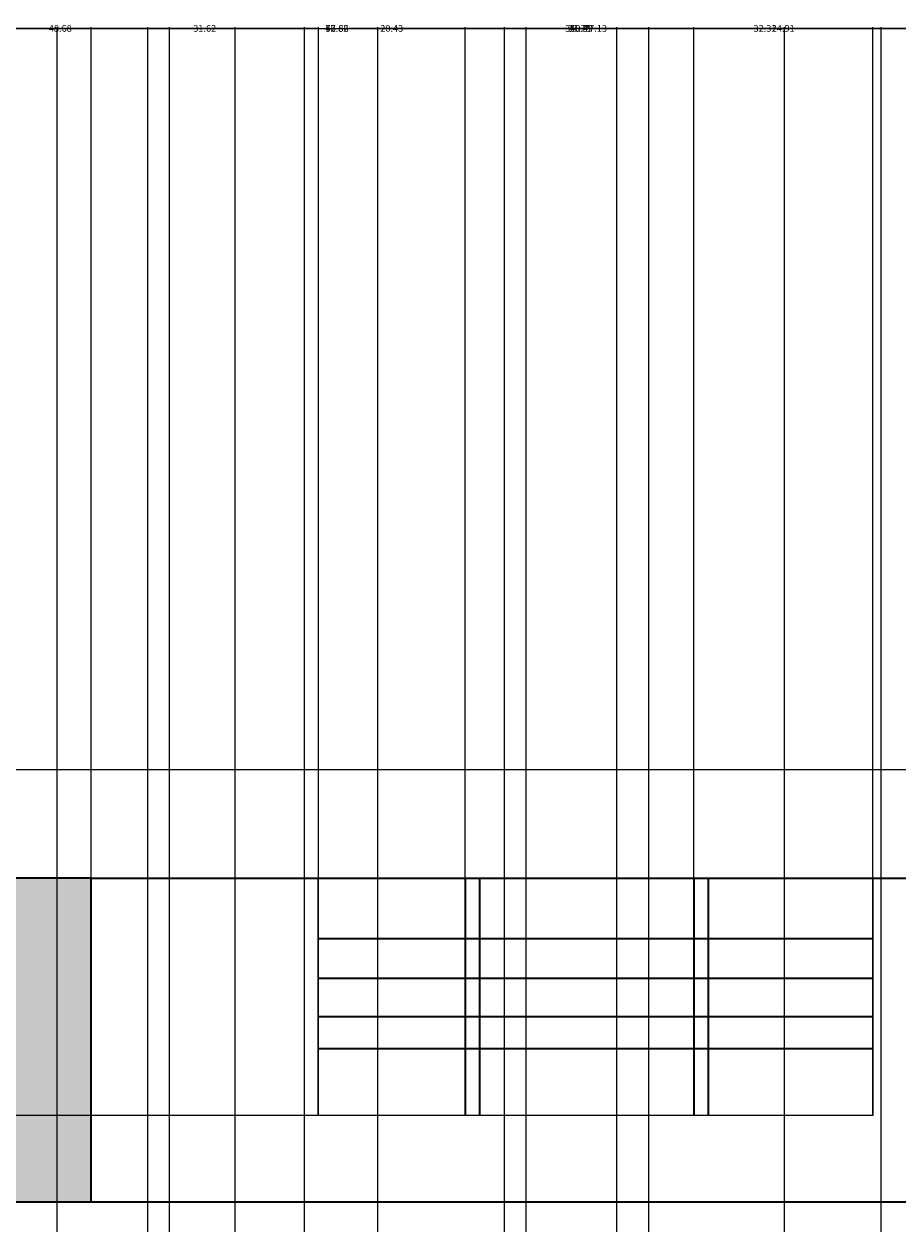
# Model space of a CAD drawing. Units: inches. Extents: x -5 to 714, y 84 to 644.
# Tile 13 of 20: x 220 to 342, y 477 to 644. Entities that reach past the tile are written whole.
import ezdxf

# ---------------------------------------------------------------- set-up
doc = ezdxf.new("R2010")
doc.units = ezdxf.units.IN
doc.header["$MEASUREMENT"] = 0
for name, color, linetype, lineweight in [('A-ANNO-DIMS', 2, 'Continuous', 18), ('A-ELEV', 7, 'Continuous', 35), ('A-ELEV-PATT', 8, 'Continuous', 13), ('A-GLAZ', 3, 'Continuous', 25)]:
    doc.layers.add(name, color=color, linetype=linetype, lineweight=lineweight)
doc.styles.get("Standard").update_dxf_attribs({"font": 'arial.ttf'})
doc.dimstyles.get("Standard").update_dxf_attribs({"dimtxt": 0.9375, "dimasz": 0.18, "dimexe": 0.18, "dimexo": 0.0625, "dimgap": 0.09, "dimtad": 0, "dimtih": 1, "dimtoh": 1, "dimdec": 4, "dimzin": 0, "dimdsep": 46, "dimlunit": 4, "dimtxsty": 'Standard', "dimcen": 0.09, "dimadec": 0, "dimazin": 0, "dimtfac": 1, "dimtdec": 4, "dimtofl": 0, "dimtmove": 0, "dimatfit": 3, "dimfxl": 1, "dimtolj": 1, "dimtzin": 0, "dimarcsym": 0})

# ---------------------------------------------------------------- blocks, each defined once
blk = doc.blocks.new('*D11')
at = {"layer": 'A-ANNO-DIMS', "color": 0, "lineweight": -2, "transparency": 16777216}
for p, q in [((198.38, 525.26), (198.38, 643.61)), ((198.56, 643.43), (211.83, 643.43)), ((229.18, 643.43), (215.91, 643.43)), ((229.36, 525.26), (229.36, 643.61))]:
    blk.add_line(p, q, dxfattribs=at)
at = {"layer": 'A-ANNO-DIMS', "color": 0, "transparency": 16777216}
for points in [[(198.56, 643.46), (198.56, 643.4), (198.38, 643.43)], [(229.18, 643.46), (229.18, 643.4), (229.36, 643.43)]]:
    blk.add_solid(points, dxfattribs=at)
at = {"layer": 'Defpoints', "color": 0, "transparency": 16777216}
for p in [(229.36, 643.43), (198.38, 525.19), (229.36, 525.19)]:
    blk.add_point(p, dxfattribs=at)
at = {"layer": 'A-ANNO-DIMS', "color": 0, "transparency": 16777216, "insert": (213.87, 643.43), "char_height": 0.938, "attachment_point": 5}
blk.add_mtext('\\A1;30.975', dxfattribs=at)
blk = doc.blocks.new('*D12')
at = {"layer": 'A-ANNO-DIMS', "color": 0, "lineweight": -2, "transparency": 16777216}
for p, q in [((229.36, 525.26), (229.36, 643.61)), ((229.54, 643.43), (243.5, 643.43)), ((260.8, 643.43), (246.83, 643.43)), ((260.98, 525.26), (260.98, 643.61))]:
    blk.add_line(p, q, dxfattribs=at)
at = {"layer": 'A-ANNO-DIMS', "color": 0, "transparency": 16777216}
for points in [[(229.54, 643.46), (229.54, 643.4), (229.36, 643.43)], [(260.8, 643.46), (260.8, 643.4), (260.98, 643.43)]]:
    blk.add_solid(points, dxfattribs=at)
at = {"layer": 'Defpoints', "color": 0, "transparency": 16777216}
for p in [(260.98, 643.43), (229.36, 525.19), (260.98, 525.19)]:
    blk.add_point(p, dxfattribs=at)
at = {"layer": 'A-ANNO-DIMS', "color": 0, "transparency": 16777216, "insert": (245.17, 643.43), "char_height": 0.938, "attachment_point": 5}
blk.add_mtext('\\A1;31.62', dxfattribs=at)
blk = doc.blocks.new('*D13')
at = {"layer": 'A-ANNO-DIMS', "color": 0, "lineweight": -2, "transparency": 16777216}
for p, q in [((260.98, 525.26), (260.98, 643.61)), ((261.16, 643.43), (297.87, 643.43)), ((337.93, 643.43), (301.21, 643.43)), ((338.11, 525.26), (338.11, 643.61))]:
    blk.add_line(p, q, dxfattribs=at)
at = {"layer": 'A-ANNO-DIMS', "color": 0, "transparency": 16777216}
for points in [[(261.16, 643.46), (261.16, 643.4), (260.98, 643.43)], [(337.93, 643.46), (337.93, 643.4), (338.11, 643.43)]]:
    blk.add_solid(points, dxfattribs=at)
at = {"layer": 'Defpoints', "color": 0, "transparency": 16777216}
for p in [(338.11, 643.43), (260.98, 525.19), (338.11, 525.19)]:
    blk.add_point(p, dxfattribs=at)
at = {"layer": 'A-ANNO-DIMS', "color": 0, "transparency": 16777216, "insert": (299.54, 643.43), "char_height": 0.938, "attachment_point": 5}
blk.add_mtext('\\A1;77.13', dxfattribs=at)
blk = doc.blocks.new('*D14')
at = {"layer": 'A-ANNO-DIMS', "color": 0, "lineweight": -2, "transparency": 16777216}
for p, q in [((338.11, 525.26), (338.11, 643.61)), ((338.29, 643.43), (349.15, 643.43)), ((364.1, 643.43), (353.24, 643.43)), ((364.28, 525.26), (364.28, 643.61))]:
    blk.add_line(p, q, dxfattribs=at)
at = {"layer": 'A-ANNO-DIMS', "color": 0, "transparency": 16777216}
for points in [[(338.29, 643.46), (338.29, 643.4), (338.11, 643.43)], [(364.1, 643.46), (364.1, 643.4), (364.28, 643.43)]]:
    blk.add_solid(points, dxfattribs=at)
at = {"layer": 'Defpoints', "color": 0, "transparency": 16777216}
for p in [(364.28, 643.43), (338.11, 525.19), (364.28, 525.19)]:
    blk.add_point(p, dxfattribs=at)
at = {"layer": 'A-ANNO-DIMS', "color": 0, "transparency": 16777216, "insert": (351.19, 643.43), "char_height": 0.938, "attachment_point": 5}
blk.add_mtext('\\A1;26.175', dxfattribs=at)
blk = doc.blocks.new('*D16')
at = {"layer": 'A-ANNO-DIMS', "color": 0, "lineweight": -2, "transparency": 16777216}
for p, q in [((364.22, 540.29), (-2.74, 540.29)), ((-2.56, 540.11), (-2.56, 510.8)), ((-2.56, 480.35), (-2.56, 509.66)), ((364.22, 480.17), (-2.74, 480.17))]:
    blk.add_line(p, q, dxfattribs=at)
at = {"layer": 'A-ANNO-DIMS', "color": 0, "transparency": 16777216}
for points in [[(-2.59, 540.11), (-2.53, 540.11), (-2.56, 540.29)], [(-2.59, 480.35), (-2.53, 480.35), (-2.56, 480.17)]]:
    blk.add_solid(points, dxfattribs=at)
at = {"layer": 'Defpoints', "color": 0, "transparency": 16777216}
for p in [(-2.56, 540.29), (364.28, 540.29), (364.28, 480.17)]:
    blk.add_point(p, dxfattribs=at)
at = {"layer": 'A-ANNO-DIMS', "color": 0, "transparency": 16777216, "insert": (-2.56, 510.23), "char_height": 0.938, "attachment_point": 5}
blk.add_mtext('\\A1;60.11', dxfattribs=at)
blk = doc.blocks.new('*D17')
at = {"layer": 'A-ANNO-DIMS', "color": 0, "lineweight": -2, "transparency": 16777216}
for p, q in [((338.04, 525.19), (-2.74, 525.19)), ((-2.56, 525.01), (-2.56, 509.25)), ((-2.56, 492.35), (-2.56, 508.11)), ((338.04, 492.17), (-2.74, 492.17))]:
    blk.add_line(p, q, dxfattribs=at)
at = {"layer": 'A-ANNO-DIMS', "color": 0, "transparency": 16777216}
for points in [[(-2.59, 525.01), (-2.53, 525.01), (-2.56, 525.19)], [(-2.59, 492.35), (-2.53, 492.35), (-2.56, 492.17)]]:
    blk.add_solid(points, dxfattribs=at)
at = {"layer": 'Defpoints', "color": 0, "transparency": 16777216}
for p in [(-2.56, 525.19), (338.11, 525.19), (338.11, 492.17)]:
    blk.add_point(p, dxfattribs=at)
at = {"layer": 'A-ANNO-DIMS', "color": 0, "transparency": 16777216, "insert": (-2.56, 508.68), "char_height": 0.938, "attachment_point": 5}
blk.add_mtext('\\A1;33.03', dxfattribs=at)
blk = doc.blocks.new('*D18')
at = {"layer": 'A-ANNO-DIMS', "color": 0, "lineweight": -2, "transparency": 16777216}
for p, q in [((260.98, 492.23), (260.98, 643.61)), ((261.16, 643.43), (269.51, 643.43)), ((281.23, 643.43), (272.87, 643.43)), ((281.41, 492.23), (281.41, 643.61))]:
    blk.add_line(p, q, dxfattribs=at)
at = {"layer": 'A-ANNO-DIMS', "color": 0, "transparency": 16777216}
for points in [[(261.16, 643.46), (261.16, 643.4), (260.98, 643.43)], [(281.23, 643.46), (281.23, 643.4), (281.41, 643.43)]]:
    blk.add_solid(points, dxfattribs=at)
at = {"layer": 'Defpoints', "color": 0, "transparency": 16777216}
for p in [(281.41, 643.43), (260.98, 492.17), (281.41, 492.17)]:
    blk.add_point(p, dxfattribs=at)
at = {"layer": 'A-ANNO-DIMS', "color": 0, "transparency": 16777216, "insert": (271.19, 643.43), "char_height": 0.938, "attachment_point": 5}
blk.add_mtext('\\A1;20.43', dxfattribs=at)
blk = doc.blocks.new('*D19')
at = {"layer": 'A-ANNO-DIMS', "color": 0, "lineweight": -2, "transparency": 16777216}
for p, q in [((281.41, 492.23), (281.41, 643.61)), ((281.59, 643.43), (295.63, 643.43)), ((313.02, 643.43), (298.98, 643.43)), ((313.2, 492.23), (313.2, 643.61))]:
    blk.add_line(p, q, dxfattribs=at)
at = {"layer": 'A-ANNO-DIMS', "color": 0, "transparency": 16777216}
for points in [[(281.59, 643.46), (281.59, 643.4), (281.41, 643.43)], [(313.02, 643.46), (313.02, 643.4), (313.2, 643.43)]]:
    blk.add_solid(points, dxfattribs=at)
at = {"layer": 'Defpoints', "color": 0, "transparency": 16777216}
for p in [(313.2, 643.43), (281.41, 492.17), (313.2, 492.17)]:
    blk.add_point(p, dxfattribs=at)
at = {"layer": 'A-ANNO-DIMS', "color": 0, "transparency": 16777216, "insert": (297.3, 643.43), "char_height": 0.938, "attachment_point": 5}
blk.add_mtext('\\A1;31.79', dxfattribs=at)
blk = doc.blocks.new('*D20')
at = {"layer": 'A-ANNO-DIMS', "color": 0, "lineweight": -2, "transparency": 16777216}
for p, q in [((313.2, 492.23), (313.2, 643.61)), ((313.38, 643.43), (324.06, 643.43)), ((337.93, 643.43), (327.24, 643.43)), ((338.11, 492.23), (338.11, 643.61))]:
    blk.add_line(p, q, dxfattribs=at)
at = {"layer": 'A-ANNO-DIMS', "color": 0, "transparency": 16777216}
for points in [[(313.38, 643.46), (313.38, 643.4), (313.2, 643.43)], [(337.93, 643.46), (337.93, 643.4), (338.11, 643.43)]]:
    blk.add_solid(points, dxfattribs=at)
at = {"layer": 'Defpoints', "color": 0, "transparency": 16777216}
for p in [(338.11, 643.43), (313.2, 492.17), (338.11, 492.17)]:
    blk.add_point(p, dxfattribs=at)
at = {"layer": 'A-ANNO-DIMS', "color": 0, "transparency": 16777216, "insert": (325.65, 643.43), "char_height": 0.938, "attachment_point": 5}
blk.add_mtext('\\A1;24.91', dxfattribs=at)
blk = doc.blocks.new('*D23')
at = {"layer": 'A-ANNO-DIMS', "color": 0, "lineweight": -2, "transparency": 16777216}
for p, q in [((229.3, 525.19), (-2.74, 525.19)), ((-2.56, 525.01), (-2.56, 503.25)), ((-2.56, 480.35), (-2.56, 502.11)), ((229.3, 480.17), (-2.74, 480.17))]:
    blk.add_line(p, q, dxfattribs=at)
at = {"layer": 'A-ANNO-DIMS', "color": 0, "transparency": 16777216}
for points in [[(-2.59, 525.01), (-2.53, 525.01), (-2.56, 525.19)], [(-2.59, 480.35), (-2.53, 480.35), (-2.56, 480.17)]]:
    blk.add_solid(points, dxfattribs=at)
at = {"layer": 'Defpoints', "color": 0, "transparency": 16777216}
for p in [(-2.56, 525.19), (229.36, 525.19), (229.36, 480.17)]:
    blk.add_point(p, dxfattribs=at)
at = {"layer": 'A-ANNO-DIMS', "color": 0, "transparency": 16777216, "insert": (-2.56, 502.68), "char_height": 0.938, "attachment_point": 5}
blk.add_mtext('\\A1;45.02', dxfattribs=at)
blk = doc.blocks.new('*D24')
at = {"layer": 'A-ANNO-DIMS', "color": 0, "lineweight": -2, "transparency": 16777216}
for p, q in [((126.73, 480.23), (126.73, 643.61)), ((126.91, 643.43), (295.25, 643.43)), ((466.92, 643.43), (298.58, 643.43)), ((467.1, 480.23), (467.1, 643.61))]:
    blk.add_line(p, q, dxfattribs=at)
at = {"layer": 'A-ANNO-DIMS', "color": 0, "transparency": 16777216}
for points in [[(126.91, 643.46), (126.91, 643.4), (126.73, 643.43)], [(466.92, 643.46), (466.92, 643.4), (467.1, 643.43)]]:
    blk.add_solid(points, dxfattribs=at)
at = {"layer": 'Defpoints', "color": 0, "transparency": 16777216}
for p in [(467.1, 643.43), (126.73, 480.17), (467.1, 480.17)]:
    blk.add_point(p, dxfattribs=at)
at = {"layer": 'A-ANNO-DIMS', "color": 0, "transparency": 16777216, "insert": (296.91, 643.43), "char_height": 0.938, "attachment_point": 5}
blk.add_mtext('\\A1;340.4', dxfattribs=at)
blk = doc.blocks.new('*D31')
at = {"layer": 'A-ANNO-DIMS', "color": 0, "lineweight": -2, "transparency": 16777216}
for p, q in [((135.73, 345.26), (135.73, 643.61)), ((135.91, 643.43), (184.51, 643.43)), ((237.09, 643.43), (188.49, 643.43)), ((237.27, 345.26), (237.27, 643.61))]:
    blk.add_line(p, q, dxfattribs=at)
at = {"layer": 'A-ANNO-DIMS', "color": 0, "transparency": 16777216}
for points in [[(135.91, 643.46), (135.91, 643.4), (135.73, 643.43)], [(237.09, 643.46), (237.09, 643.4), (237.27, 643.43)]]:
    blk.add_solid(points, dxfattribs=at)
at = {"layer": 'Defpoints', "color": 0, "transparency": 16777216}
for p in [(237.27, 643.43), (135.73, 345.19), (237.27, 345.19)]:
    blk.add_point(p, dxfattribs=at)
at = {"layer": 'A-ANNO-DIMS', "color": 0, "transparency": 16777216, "insert": (186.5, 643.43), "char_height": 0.938, "attachment_point": 5}
blk.add_mtext('\\A1;101.54', dxfattribs=at)
blk = doc.blocks.new('*D32')
at = {"layer": 'A-ANNO-DIMS', "color": 0, "lineweight": -2, "transparency": 16777216}
for p, q in [((237.27, 417.15), (237.27, 643.61)), ((237.45, 643.43), (261.91, 643.43)), ((289.7, 643.43), (265.24, 643.43)), ((289.88, 417.15), (289.88, 643.61))]:
    blk.add_line(p, q, dxfattribs=at)
at = {"layer": 'A-ANNO-DIMS', "color": 0, "transparency": 16777216}
for points in [[(237.45, 643.46), (237.45, 643.4), (237.27, 643.43)], [(289.7, 643.46), (289.7, 643.4), (289.88, 643.43)]]:
    blk.add_solid(points, dxfattribs=at)
at = {"layer": 'Defpoints', "color": 0, "transparency": 16777216}
for p in [(289.88, 643.43), (237.27, 417.09), (289.88, 417.09)]:
    blk.add_point(p, dxfattribs=at)
at = {"layer": 'A-ANNO-DIMS', "color": 0, "transparency": 16777216, "insert": (263.57, 643.43), "char_height": 0.938, "attachment_point": 5}
blk.add_mtext('\\A1;52.62', dxfattribs=at)
blk = doc.blocks.new('*D33')
at = {"layer": 'A-ANNO-DIMS', "color": 0, "lineweight": -2, "transparency": 16777216}
for p, q in [((240.27, 348.26), (240.27, 643.61)), ((240.45, 643.43), (261.89, 643.43)), ((286.7, 643.43), (265.26, 643.43)), ((286.88, 348.26), (286.88, 643.61))]:
    blk.add_line(p, q, dxfattribs=at)
at = {"layer": 'A-ANNO-DIMS', "color": 0, "transparency": 16777216}
for points in [[(240.45, 643.46), (240.45, 643.4), (240.27, 643.43)], [(286.7, 643.46), (286.7, 643.4), (286.88, 643.43)]]:
    blk.add_solid(points, dxfattribs=at)
at = {"layer": 'Defpoints', "color": 0, "transparency": 16777216}
for p in [(286.88, 643.43), (240.27, 348.19), (286.88, 348.19)]:
    blk.add_point(p, dxfattribs=at)
at = {"layer": 'A-ANNO-DIMS', "color": 0, "transparency": 16777216, "insert": (263.57, 643.43), "char_height": 0.938, "attachment_point": 5}
blk.add_mtext('\\A1;46.62', dxfattribs=at)
blk = doc.blocks.new('*D36')
at = {"layer": 'A-ANNO-DIMS', "color": 0, "lineweight": -2, "transparency": 16777216}
for p, q in [((224.64, 426.51), (224.64, 643.61)), ((224.82, 643.43), (261.91, 643.43)), ((302.32, 643.43), (265.24, 643.43)), ((302.5, 426.51), (302.5, 643.61))]:
    blk.add_line(p, q, dxfattribs=at)
at = {"layer": 'A-ANNO-DIMS', "color": 0, "transparency": 16777216}
for points in [[(224.82, 643.46), (224.82, 643.4), (224.64, 643.43)], [(302.32, 643.46), (302.32, 643.4), (302.5, 643.43)]]:
    blk.add_solid(points, dxfattribs=at)
at = {"layer": 'Defpoints', "color": 0, "transparency": 16777216}
for p in [(302.5, 643.43), (224.64, 426.45), (302.5, 426.45)]:
    blk.add_point(p, dxfattribs=at)
at = {"layer": 'A-ANNO-DIMS', "color": 0, "transparency": 16777216, "insert": (263.57, 643.43), "char_height": 0.938, "attachment_point": 5}
blk.add_mtext('\\A1;77.86', dxfattribs=at)
blk = doc.blocks.new('*D51')
at = {"layer": 'A-ANNO-DIMS', "color": 0, "lineweight": -2, "transparency": 16777216}
for p, q in [((200.74, 201.26), (200.74, 643.61)), ((200.92, 643.43), (223.39, 643.43)), ((249.24, 643.43), (226.77, 643.43)), ((249.42, 201.26), (249.42, 643.61))]:
    blk.add_line(p, q, dxfattribs=at)
at = {"layer": 'A-ANNO-DIMS', "color": 0, "transparency": 16777216}
for points in [[(200.92, 643.46), (200.92, 643.4), (200.74, 643.43)], [(249.24, 643.46), (249.24, 643.4), (249.42, 643.43)]]:
    blk.add_solid(points, dxfattribs=at)
at = {"layer": 'Defpoints', "color": 0, "transparency": 16777216}
for p in [(249.42, 643.43), (200.74, 201.19), (249.42, 201.19)]:
    blk.add_point(p, dxfattribs=at)
at = {"layer": 'A-ANNO-DIMS', "color": 0, "transparency": 16777216, "insert": (225.08, 643.43), "char_height": 0.938, "attachment_point": 5}
blk.add_mtext('\\A1;48.68', dxfattribs=at)
blk = doc.blocks.new('*D54')
at = {"layer": 'A-ANNO-DIMS', "color": 0, "lineweight": -2, "transparency": 16777216}
for p, q in [((259.07, 315.16), (259.07, 643.61)), ((259.25, 643.43), (424.21, 643.43)), ((593.25, 643.43), (428.28, 643.43)), ((593.43, 315.16), (593.43, 643.61))]:
    blk.add_line(p, q, dxfattribs=at)
at = {"layer": 'A-ANNO-DIMS', "color": 0, "transparency": 16777216}
for points in [[(259.25, 643.46), (259.25, 643.4), (259.07, 643.43)], [(593.25, 643.46), (593.25, 643.4), (593.43, 643.43)]]:
    blk.add_solid(points, dxfattribs=at)
at = {"layer": 'Defpoints', "color": 0, "transparency": 16777216}
for p in [(593.43, 643.43), (259.07, 315.1), (593.43, 315.1)]:
    blk.add_point(p, dxfattribs=at)
at = {"layer": 'A-ANNO-DIMS', "color": 0, "transparency": 16777216, "insert": (426.25, 643.43), "char_height": 0.938, "attachment_point": 5}
blk.add_mtext('\\A1;334.36', dxfattribs=at)
blk = doc.blocks.new('*D60')
at = {"layer": 'A-ANNO-DIMS', "color": 0, "lineweight": -2, "transparency": 16777216}
for p, q in [((269.24, 277.11), (269.24, 643.61)), ((269.42, 643.43), (295.86, 643.43)), ((325.65, 643.43), (299.21, 643.43)), ((325.83, 266.06), (325.83, 643.61))]:
    blk.add_line(p, q, dxfattribs=at)
at = {"layer": 'A-ANNO-DIMS', "color": 0, "transparency": 16777216}
for points in [[(269.42, 643.46), (269.42, 643.4), (269.24, 643.43)], [(325.65, 643.46), (325.65, 643.4), (325.83, 643.43)]]:
    blk.add_solid(points, dxfattribs=at)
at = {"layer": 'Defpoints', "color": 0, "transparency": 16777216}
for p in [(325.83, 643.43), (269.24, 277.05), (325.83, 266)]:
    blk.add_point(p, dxfattribs=at)
at = {"layer": 'A-ANNO-DIMS', "color": 0, "transparency": 16777216, "insert": (297.54, 643.43), "char_height": 0.938, "attachment_point": 5}
blk.add_mtext('\\A1;56.59', dxfattribs=at)
blk = doc.blocks.new('*D61')
at = {"layer": 'A-ANNO-DIMS', "color": 0, "lineweight": -2, "transparency": 16777216}
for p, q in [((325.83, 266.06), (325.83, 643.61)), ((326.01, 643.43), (364.93, 643.43)), ((407.2, 643.43), (368.28, 643.43)), ((407.38, 266.06), (407.38, 643.61))]:
    blk.add_line(p, q, dxfattribs=at)
at = {"layer": 'A-ANNO-DIMS', "color": 0, "transparency": 16777216}
for points in [[(326.01, 643.46), (326.01, 643.4), (325.83, 643.43)], [(407.2, 643.46), (407.2, 643.4), (407.38, 643.43)]]:
    blk.add_solid(points, dxfattribs=at)
at = {"layer": 'Defpoints', "color": 0, "transparency": 16777216}
for p in [(407.38, 643.43), (325.83, 266), (407.38, 266)]:
    blk.add_point(p, dxfattribs=at)
at = {"layer": 'A-ANNO-DIMS', "color": 0, "transparency": 16777216, "insert": (366.61, 643.43), "char_height": 0.938, "attachment_point": 5}
blk.add_mtext('\\A1;81.55', dxfattribs=at)
blk = doc.blocks.new('*D83')
at = {"layer": 'A-ANNO-DIMS', "color": 0, "lineweight": -2, "transparency": 16777216}
for p, q in [((306.96, 144.93), (306.96, 643.61)), ((307.14, 643.43), (321.53, 643.43)), ((339.09, 643.43), (324.69, 643.43)), ((339.27, 144.93), (339.27, 643.61))]:
    blk.add_line(p, q, dxfattribs=at)
at = {"layer": 'A-ANNO-DIMS', "color": 0, "transparency": 16777216}
for points in [[(307.14, 643.46), (307.14, 643.4), (306.96, 643.43)], [(339.09, 643.46), (339.09, 643.4), (339.27, 643.43)]]:
    blk.add_solid(points, dxfattribs=at)
at = {"layer": 'Defpoints', "color": 0, "transparency": 16777216}
for p in [(339.27, 643.43), (306.96, 144.86), (339.27, 144.86)]:
    blk.add_point(p, dxfattribs=at)
at = {"layer": 'A-ANNO-DIMS', "color": 0, "transparency": 16777216, "insert": (323.11, 643.43), "char_height": 0.938, "attachment_point": 5}
blk.add_mtext('\\A1;32.31', dxfattribs=at)

msp = doc.modelspace()

# ---------------------------------------------------------------- hatches: boundary and pattern name
at = {"layer": 'A-ELEV-PATT', "transparency": 33554687}
h = msp.add_hatch(color=256, dxfattribs=at)
h.dxf.hatch_style = 1
h.paths.add_polyline_path([(188.3677, 525.1928), (67.9893, 525.1928), (67.9893, 489.1928), (67.9893, 345.1928), (126.7303, 345.1928), (126.7303, 480.1709), (229.3575, 480.1709), (229.3575, 525.1928), (212.6043, 525.1928), (212.6043, 482.7164), (211.0019, 482.7164), (211.0019, 525.1928), (207.6919, 525.1928), (199.9852, 525.1928), (199.9852, 482.7164), (198.3828, 482.7164), (198.3828, 525.1928), (189.9701, 525.1928), (189.9701, 482.7164), (188.3677, 482.7164)])
h.paths.add_polyline_path([(121.3589, 336.2066), (75.5048, 336.2066), (75.5048, 319.345), (121.3589, 319.345)])
h.paths.add_polyline_path([(121.3589, 319.345), (75.5048, 319.345), (75.5048, 302.3045), (121.3589, 302.3045)])
h.paths.add_polyline_path([(121.3589, 302.3045), (75.5048, 302.3045), (75.5048, 282.8561), (121.3589, 282.8561)])
h.paths.add_polyline_path([(121.3589, 282.8561), (75.5048, 282.8561), (75.5048, 261.5556), (121.3589, 261.5556)])
h.paths.add_polyline_path([(121.3589, 261.5556), (75.5048, 261.5556), (75.5048, 243.7009), (121.3589, 243.7009)])
h.paths.add_polyline_path([(121.3589, 243.7009), (75.5048, 243.7009), (75.5048, 223.5117), (121.3589, 223.5117)])
h.paths.add_polyline_path([(121.3589, 223.5117), (75.5048, 223.5117), (75.5048, 212.5836), (121.3589, 212.5836)])
h.paths.add_polyline_path([(121.3589, 212.5836), (75.5048, 212.5836), (75.5048, 201.1928), (121.3589, 201.1928)])
h.paths.add_polyline_path([(179.9335, 201.1928), (30.1395, 201.1928), (30.1395, 198.7054), (179.9335, 198.7054)])
h.paths.add_polyline_path([(187.6349, 201.1928), (179.9335, 201.1928), (179.9335, 198.7054), (179.9335, 141.1928), (269.2446, 141.1928), (269.2446, 201.1928), (263.4349, 201.1928), (263.4349, 152.1176), (187.6349, 152.1176)])
h.paths.add_polyline_path([(269.2446, 277.0513), (269.2446, 287.501), (269.2446, 306.6286), (578.0915, 306.6286), (578.0915, 201.1928), (593.428, 201.1928), (593.428, 315.0968), (584.4202, 315.0968), (259.0665, 315.0968), (259.0665, 201.1928), (263.4349, 201.1928), (269.2446, 201.1928)])

# ---------------------------------------------------------------- linework, layer by layer
at = {"layer": 'A-ELEV'}
for p, q in [((229.3575, 525.1928), (207.6919, 525.1928)), ((229.3575, 480.1709), (229.3575, 525.1928)), ((229.3575, 525.1928), (364.2809, 525.1928)), ((281.4098, 525.1928), (281.4098, 492.1651)), ((283.4098, 525.1928), (283.4098, 492.1651)), ((313.1984, 525.1928), (313.1984, 492.1651)), ((315.1984, 525.1928), (315.1984, 492.1651)), ((260.9786, 516.8026), (338.106, 516.8026)), ((260.9786, 511.2941), (338.106, 511.2941)), ((260.9786, 505.9633), (338.106, 505.9633)), ((260.9786, 501.521), (338.106, 501.521)), ((126.7303, 480.1709), (229.3575, 480.1709)), ((229.3575, 480.1709), (467.0994, 480.1709))]:
    msp.add_line(p, q, dxfattribs=at)
at = {"layer": 'A-GLAZ'}
msp.add_lwpolyline([(260.9786, 525.1928), (338.106, 525.1928), (338.106, 492.1651), (260.9786, 492.1651)], close=True, dxfattribs=at)

# ---------------------------------------------------------------- dimensions: what is measured, and where the dimension line sits
at = {"layer": 'A-ANNO-DIMS'}
for base, p1, p2, override, picture, middle in [((467.0994, 643.4276), (126.7303, 480.1709), (467.0994, 480.1709), {"dimdec": 1, "dimlfac": 1, "dimrnd": 0, "dimzin": 0, "dimdsep": 46, "dimlunit": 2}, '*D24', (296.9148, 643.4276)), ((237.2654, 643.4276), (135.7303, 345.1928), (237.2654, 345.1928), {"dimdec": 2, "dimlfac": 1, "dimrnd": 0, "dimzin": 0, "dimdsep": 46, "dimlunit": 2}, '*D31', (186.4978, 643.4276)), ((229.3575, 643.4276), (198.3828, 525.1928), (229.3575, 525.1928), {"dimdec": 3, "dimlfac": 1, "dimrnd": 0, "dimzin": 0, "dimdsep": 46, "dimlunit": 2}, '*D11', (213.8702, 643.4276)), ((249.4181, 643.4276), (200.7361, 201.1928), (249.4181, 201.1928), {"dimdec": 2, "dimlfac": 1, "dimrnd": 0, "dimzin": 0, "dimdsep": 46, "dimlunit": 2}, '*D51', (225.0771, 643.4276)), ((302.5023, 643.4276), (224.6446, 426.4485), (302.5023, 426.4485), {"dimdec": 2, "dimlfac": 1, "dimrnd": 0, "dimzin": 0, "dimdsep": 46, "dimlunit": 2}, '*D36', (263.5734, 643.4276)), ((260.9786, 643.4276), (229.3575, 525.1928), (260.9786, 525.1928), {"dimdec": 2, "dimlfac": 1, "dimrnd": 0, "dimzin": 0, "dimdsep": 46, "dimlunit": 2}, '*D12', (245.1681, 643.4276)), ((289.8815, 643.4276), (237.2654, 417.0908), (289.8815, 417.0908), {"dimdec": 2, "dimlfac": 1, "dimrnd": 0, "dimzin": 0, "dimdsep": 46, "dimlunit": 2}, '*D32', (263.5734, 643.4276)), ((286.8815, 643.4276), (240.2654, 348.1928), (286.8815, 348.1928), {"dimdec": 2, "dimlfac": 1, "dimrnd": 0, "dimzin": 0, "dimdsep": 46, "dimlunit": 2}, '*D33', (263.5734, 643.4276)), ((593.428, 643.4276), (259.0665, 315.0968), (593.428, 315.0968), {"dimdec": 2, "dimlfac": 1, "dimrnd": 0, "dimzin": 0, "dimdsep": 46, "dimlunit": 2}, '*D54', (426.2472, 643.4276)), ((338.106, 643.4276), (260.9786, 525.1928), (338.106, 525.1928), {"dimdec": 2, "dimlfac": 1, "dimrnd": 0, "dimzin": 0, "dimdsep": 46, "dimlunit": 2}, '*D13', (299.5423, 643.4276)), ((281.4098, 643.4276), (260.9786, 492.1651), (281.4098, 492.1651), {"dimdec": 2, "dimlfac": 1, "dimrnd": 0, "dimzin": 0, "dimdsep": 46, "dimlunit": 2}, '*D18', (271.1942, 643.4276)), ((325.8305, 643.4276), (269.2446, 277.0513), (325.8305, 266.0021), {"dimdec": 2, "dimlfac": 1, "dimrnd": 0, "dimzin": 0, "dimdsep": 46, "dimlunit": 2}, '*D60', (297.5375, 643.4276)), ((313.1984, 643.4276), (281.4098, 492.1651), (313.1984, 492.1651), {"dimdec": 2, "dimlfac": 1, "dimrnd": 0, "dimzin": 0, "dimdsep": 46, "dimlunit": 2}, '*D19', (297.3041, 643.4276)), ((339.2672, 643.4276), (306.958, 144.8639), (339.2672, 144.8639), {"dimdec": 2, "dimlfac": 1, "dimrnd": 0, "dimzin": 0, "dimdsep": 46, "dimlunit": 2}, '*D83', (323.1126, 643.4276)), ((338.106, 643.4276), (313.1984, 492.1651), (338.106, 492.1651), {"dimdec": 2, "dimlfac": 1, "dimrnd": 0, "dimzin": 0, "dimdsep": 46, "dimlunit": 2}, '*D20', (325.6522, 643.4276)), ((407.3813, 643.4276), (325.8305, 266.0021), (407.3813, 266.0021), {"dimdec": 2, "dimlfac": 1, "dimrnd": 0, "dimzin": 0, "dimdsep": 46, "dimlunit": 2}, '*D61', (366.6059, 643.4276)), ((364.2809, 643.4276), (338.106, 525.1928), (364.2809, 525.1928), {"dimdec": 3, "dimlfac": 1, "dimrnd": 0, "dimzin": 0, "dimdsep": 46, "dimlunit": 2}, '*D14', (351.1934, 643.4276))]:
    dim = msp.add_linear_dim(base=base, p1=p1, p2=p2, dimstyle='Standard', override=override, dxfattribs=at)
    dim.commit()
    dim.dimension.update_dxf_attribs({"geometry": picture, "text_midpoint": middle})
for base, p1, p2, picture, middle in [((-2.5605, 540.2857), (364.2809, 480.1709), (364.2809, 540.2857), '*D16', (-2.5605, 510.2283)), ((-2.5605, 525.1928), (338.106, 492.1651), (338.106, 525.1928), '*D17', (-2.5605, 508.679)), ((-2.5605, 525.1928), (229.3575, 480.1709), (229.3575, 525.1928), '*D23', (-2.5605, 502.6819))]:
    dim = msp.add_linear_dim(base=base, p1=p1, p2=p2, angle=90, dimstyle='Standard', override={"dimdec": 2, "dimlfac": 1, "dimrnd": 0, "dimzin": 0, "dimdsep": 46, "dimlunit": 2}, dxfattribs=at)
    dim.commit()
    dim.dimension.update_dxf_attribs({"geometry": picture, "text_midpoint": middle})

doc.saveas('drawing.dxf')
